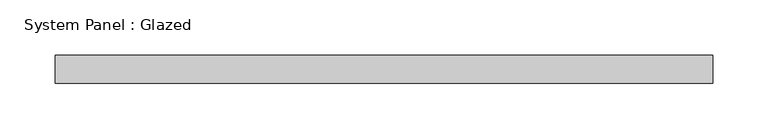
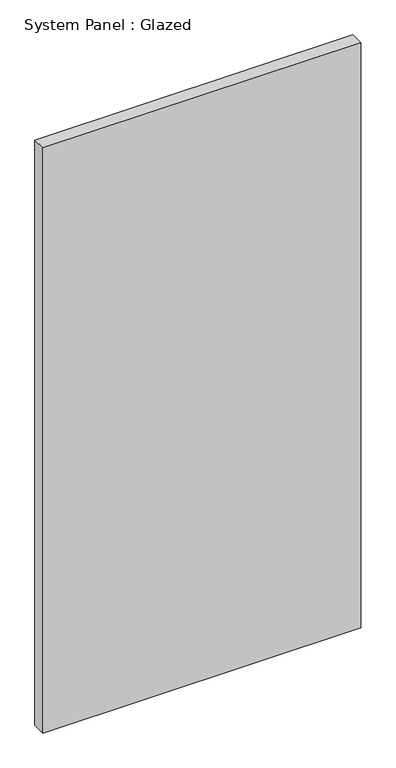
"""IFC4 building model written with IfcOpenShell, lengths in millimetres: plate geometry, System Panel : Glazed."""

from ifc_helpers import new_model, si_unit, origin, origin_with_axes, place, context, project, spatial, polyline, outline, extrude, source, transform, mapped, element, save


def system_panel_glazed_88916357(model_context):
    return source(origin(), model_context, "Body", "SweptSolid", [
        extrude(outline(polyline([(297.0061363, 19.05), (-297.0061363, 19.05), (-297.0061363, 44.45), (297.0061363, 44.45), (297.0061363, 19.05)])), origin_with_axes(), (0.0, 0.0, 1.0), 1155.7),
    ])


if __name__ == "__main__":
    model = new_model("IFC4")
    model_context = context("Model", 3, world=origin())
    ifc_project = project(units=[si_unit("LENGTHUNIT", "METRE", prefix="MILLI")], contexts=[model_context])
    site = spatial("IfcSite", under=ifc_project)
    building = spatial("IfcBuilding", under=site)
    placement = place(None, origin())
    system_panel_glazed_shape = system_panel_glazed_88916357(model_context)
    element("IfcPlate", 1, ObjectType="System Panel : Glazed", at=placement, inside=building, context=model_context, shape_type="MappedRepresentation", body=[
        mapped(system_panel_glazed_shape, transform((0.0, 0.0, 0.0), x_axis=(1.0, 0.0, 0.0), y_axis=(0.0, 1.0, 0.0), z_axis=(0.0, 0.0, 1.0))),
    ])
    save(model, "model.ifc")

# Revit data of these elements
# Type "System Panel : Glazed"
#   Construction Type Id = "GSP4R"
#   Analytic Construction = "1/8 in Pilkington single glazing"
#   Visual Light Transmittance = 0.9
#   Solar Heat Gain Coefficient = 0.86
#   Heat Transfer Coefficient (U) = 1.18115 BTU/(h·ft²·°F)
# Element 1 (IfcPlate, "System Panel : Glazed")
#   Materials on its faces: "Glass"
# Materials
#   "Glass": class "Glass", colour RGB 0 128 192, transparency 0.75, Description = "Soda Lime Glass", Cost = 0
